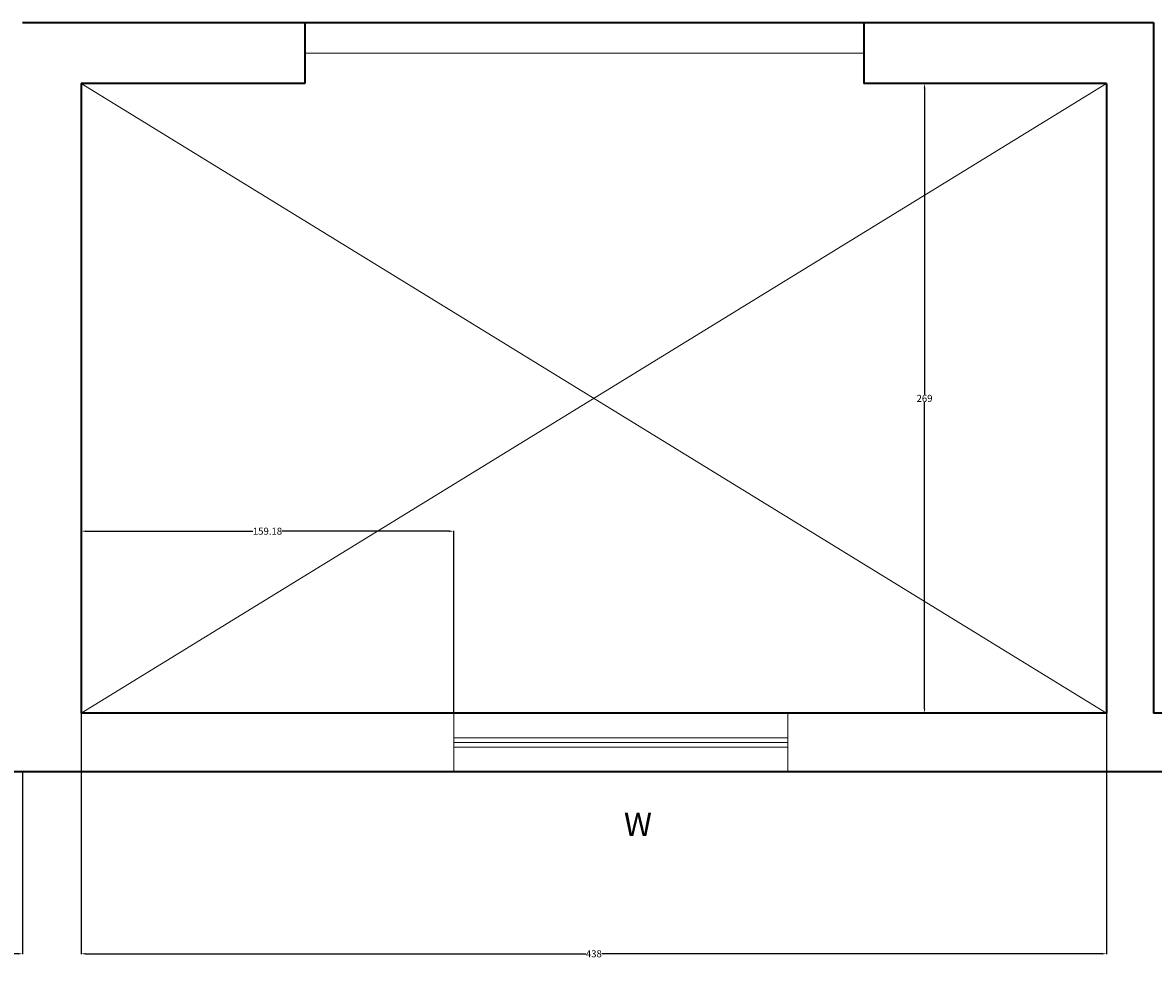
# Model space of a CAD drawing. Units: centimetres. Extents: x -121 to 3851, y -16 to 1180.
# Tile 12 of 16: x 2821 to 3304, y 16 to 416. Entities that reach past the tile are written whole.
import ezdxf

# ---------------------------------------------------------------- set-up
doc = ezdxf.new("R2010")
doc.units = ezdxf.units.CM
doc.header["$MEASUREMENT"] = 0
for name, color, linetype, lineweight in [('A-ANNO-DIMS', 2, 'Continuous', 18), ('A-ANNO-IDEN', 3, 'Continuous', 13), ('A-FLOR-HRAL', 4, 'Continuous', 18), ('A-FLOR-OPEN', 8, 'Continuous', 13), ('A-GLAZ', 4, 'Continuous', 18), ('A-WALL', 7, 'Continuous', 35)]:
    doc.layers.add(name, color=color, linetype=linetype, lineweight=lineweight)
doc.styles.get("Standard").update_dxf_attribs({"font": 'arial.ttf'})
doc.dimstyles.get("Standard").update_dxf_attribs({"dimtxt": 3, "dimasz": 2, "dimexe": 0.18, "dimexo": 0.0625, "dimgap": 0.09, "dimtad": 0, "dimtih": 1, "dimtoh": 1, "dimdec": 0, "dimzin": 0, "dimdsep": 46, "dimtxsty": 'Standard', "dimcen": 0.09, "dimadec": 0, "dimazin": 0, "dimtfac": 1, "dimtdec": 0, "dimtofl": 0, "dimtmove": 0, "dimatfit": 3, "dimfxl": 1, "dimtolj": 1, "dimtzin": 0, "dimarcsym": 0})

# ---------------------------------------------------------------- blocks, each defined once
blk = doc.blocks.new('WIN-143CM')
for p, q in [((0, 14.5), (142.63, 14.5)), ((0, 12.5), (142.63, 12.5)), ((0, 10.5), (142.63, 10.5))]:
    blk.add_line(p, q)
blk.add_lwpolyline([(0, 25), (142.63, 25), (142.63, 0), (0, 0)], close=True)
blk = doc.blocks.new('*D67')
at = {"layer": 'A-ANNO-DIMS', "color": 0, "lineweight": -2, "transparency": 16777216}
for p, q in [((2411.26, 95.66), (2411.26, 17.79)), ((2821.26, 95.66), (2821.26, 17.79)), ((2413.26, 17.97), (2612.8, 17.97)), ((2819.26, 17.97), (2619.72, 17.97))]:
    blk.add_line(p, q, dxfattribs=at)
at = {"layer": 'A-ANNO-DIMS', "color": 0, "transparency": 16777216}
for points in [[(2413.26, 18.31), (2413.26, 17.64), (2411.26, 17.97)], [(2819.26, 18.31), (2819.26, 17.64), (2821.26, 17.97)]]:
    blk.add_solid(points, dxfattribs=at)
at = {"layer": 'Defpoints', "color": 0, "transparency": 16777216}
for p in [(2411.26, 95.72), (2821.26, 95.72), (2821.26, 17.97)]:
    blk.add_point(p, dxfattribs=at)
at = {"layer": 'A-ANNO-DIMS', "color": 0, "transparency": 16777216, "insert": (2616.26, 17.97), "char_height": 3, "attachment_point": 5}
blk.add_mtext('\\A1;410', dxfattribs=at)
blk = doc.blocks.new('*D73')
at = {"layer": 'A-ANNO-DIMS', "color": 0, "lineweight": -2, "transparency": 16777216}
for p, q in [((2846.26, 120.66), (2846.26, 17.79)), ((3284.26, 120.66), (3284.26, 17.79)), ((2848.26, 17.97), (3061.8, 17.97)), ((3282.26, 17.97), (3068.73, 17.97))]:
    blk.add_line(p, q, dxfattribs=at)
at = {"layer": 'A-ANNO-DIMS', "color": 0, "transparency": 16777216}
for points in [[(2848.26, 18.31), (2848.26, 17.64), (2846.26, 17.97)], [(3282.26, 18.31), (3282.26, 17.64), (3284.26, 17.97)]]:
    blk.add_solid(points, dxfattribs=at)
at = {"layer": 'Defpoints', "color": 0, "transparency": 16777216}
for p in [(2846.26, 120.72), (3284.26, 120.72), (3284.26, 17.97)]:
    blk.add_point(p, dxfattribs=at)
at = {"layer": 'A-ANNO-DIMS', "color": 0, "transparency": 16777216, "insert": (3065.26, 17.97), "char_height": 3, "attachment_point": 5}
blk.add_mtext('\\A1;438', dxfattribs=at)
blk = doc.blocks.new('*D74')
at = {"layer": 'A-ANNO-DIMS', "color": 0, "lineweight": -2, "transparency": 16777216}
for p, q in [((3284.2, 389.72), (3206.33, 389.72)), ((3206.51, 387.72), (3206.51, 256.84)), ((3206.51, 122.72), (3206.51, 253.6)), ((3284.2, 120.72), (3206.33, 120.72))]:
    blk.add_line(p, q, dxfattribs=at)
at = {"layer": 'A-ANNO-DIMS', "color": 0, "transparency": 16777216}
for points in [[(3206.18, 387.72), (3206.85, 387.72), (3206.51, 389.72)], [(3206.18, 122.72), (3206.85, 122.72), (3206.51, 120.72)]]:
    blk.add_solid(points, dxfattribs=at)
at = {"layer": 'Defpoints', "color": 0, "transparency": 16777216}
for p in [(3206.51, 389.72), (3284.26, 389.72), (3284.26, 120.72)]:
    blk.add_point(p, dxfattribs=at)
at = {"layer": 'A-ANNO-DIMS', "color": 0, "transparency": 16777216, "insert": (3206.51, 255.22), "char_height": 3, "attachment_point": 5}
blk.add_mtext('\\A1;269', dxfattribs=at)
blk = doc.blocks.new('*D77')
at = {"layer": 'A-ANNO-DIMS', "color": 0, "lineweight": -2, "transparency": 16777216}
for p, q in [((2846.26, 120.79), (2846.26, 198.65)), ((2848.26, 198.47), (2919.67, 198.47)), ((3003.44, 198.47), (2932.03, 198.47)), ((3005.44, 120.79), (3005.44, 198.65))]:
    blk.add_line(p, q, dxfattribs=at)
at = {"layer": 'A-ANNO-DIMS', "color": 0, "transparency": 16777216}
for points in [[(2848.26, 198.81), (2848.26, 198.14), (2846.26, 198.47)], [(3003.44, 198.81), (3003.44, 198.14), (3005.44, 198.47)]]:
    blk.add_solid(points, dxfattribs=at)
at = {"layer": 'Defpoints', "color": 0, "transparency": 16777216}
for p in [(3005.44, 198.47), (2846.26, 120.72), (3005.44, 120.72)]:
    blk.add_point(p, dxfattribs=at)
at = {"layer": 'A-ANNO-DIMS', "color": 0, "transparency": 16777216, "insert": (2925.85, 198.47), "char_height": 3, "attachment_point": 5}
blk.add_mtext('\\A1;159.18', dxfattribs=at)

msp = doc.modelspace()

# ---------------------------------------------------------------- linework, layer by layer
at = {"layer": 'A-FLOR-HRAL'}
msp.add_line((2941.8345, 402.7228), (3180.608, 402.7228), dxfattribs=at)
at = {"layer": 'A-FLOR-OPEN'}
for p, q in [((2846.2642, 120.7228), (3284.2642, 389.7228)), ((2846.2642, 389.7228), (3284.2642, 120.7228))]:
    msp.add_line(p, q, dxfattribs=at)
at = {"layer": 'A-WALL'}
for p, q in [((2821.2642, 415.7228), (3180.608, 415.7228)), ((2941.8345, 415.7228), (2941.8345, 389.7228)), ((3180.608, 415.7228), (3304.2642, 415.7228)), ((3180.608, 415.7228), (3180.608, 389.7228)), ((3304.2642, 415.7228), (3304.2642, 120.7228)), ((2846.2642, 389.7228), (2846.2642, 120.7228)), ((2941.8345, 389.7228), (2846.2642, 389.7228)), ((3284.2642, 389.7228), (3180.608, 389.7228)), ((3284.2642, 389.7228), (3284.2642, 120.7228)), ((3284.2642, 120.7228), (2846.2642, 120.7228)), ((3742.2642, 120.7228), (3304.2642, 120.7228)), ((3767.2642, 95.7228), (2411.2642, 95.7228))]:
    msp.add_line(p, q, dxfattribs=at)

# ---------------------------------------------------------------- block references
at = {"layer": 'A-GLAZ'}
msp.add_blockref('WIN-143CM', (3005.4431, 95.7227), dxfattribs=at)

# ---------------------------------------------------------------- texts
at = {"layer": 'A-ANNO-IDEN', "insert": (3078.107, 78.2534), "char_height": 10, "attachment_point": 1}
msp.add_mtext_dynamic_manual_height_columns('W', width=55.718495, gutter_width=1, heights=[0], dxfattribs=at)

# ---------------------------------------------------------------- dimensions: what is measured, and where the dimension line sits
at = {"layer": 'A-ANNO-DIMS'}
for base, p1, p2, angle, override, picture, middle in [((3206.5142, 389.7228), (3284.2642, 120.7228), (3284.2642, 389.7228), 90, {"dimdec": 0, "dimlfac": 1, "dimrnd": 0, "dimzin": 0, "dimdsep": 46, "dimlunit": 2}, '*D74', (3206.5142, 255.2228)), ((3005.4431, 198.4728), (2846.2642, 120.7228), (3005.4431, 120.7228), 0, {"dimdec": 2, "dimlfac": 1, "dimrnd": 0, "dimzin": 0, "dimdsep": 46, "dimlunit": 2}, '*D77', (2925.8537, 198.4728))]:
    dim = msp.add_linear_dim(base=base, p1=p1, p2=p2, angle=angle, dimstyle='Standard', override=override, dxfattribs=at)
    dim.commit()
    dim.dimension.update_dxf_attribs({"geometry": picture, "text_midpoint": middle})
for base, p1, p2, picture, middle in [((3284.2642, 17.9728), (2846.2642, 120.7228), (3284.2642, 120.7228), '*D73', (3065.2642, 17.9728)), ((2821.2642, 17.9728), (2411.2642, 95.7228), (2821.2642, 95.7228), '*D67', (2616.2642, 17.9728))]:
    dim = msp.add_linear_dim(base=base, p1=p1, p2=p2, dimstyle='Standard', override={"dimdec": 0, "dimlfac": 1, "dimrnd": 0, "dimzin": 0, "dimdsep": 46, "dimlunit": 2}, dxfattribs=at)
    dim.commit()
    dim.dimension.update_dxf_attribs({"geometry": picture, "text_midpoint": middle})

doc.saveas('drawing.dxf')
